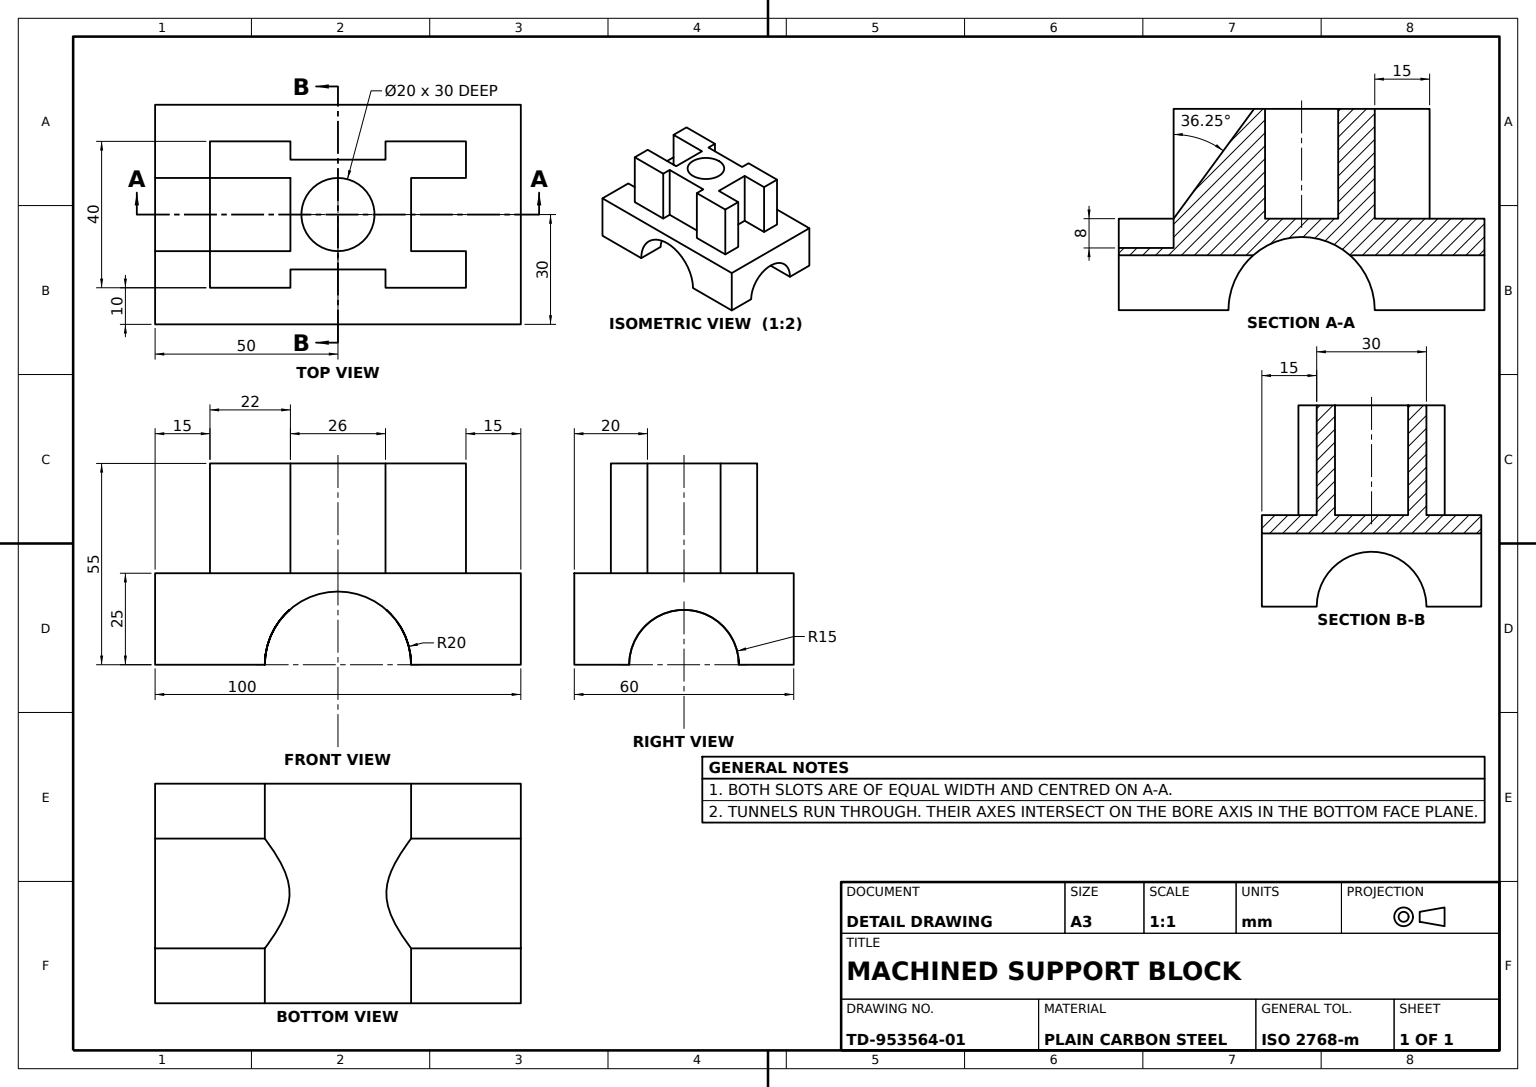
from build123d import *

# Parameters (mm, degrees)
SADDLE_BASE_BLOCK_DEPTH     = 30
THROUGH_HOLE_15_DEPTH       = 106.148704224
SLOT_CUT_DEPTH              = 15
CROSS_BOSS_PROFILE_SKETCH_R = 10
CROSS_BOSS_DEPTH            = 30
UPPER_PAD_SKETCH_W          = 20
UPPER_PAD_SKETCH_H          = 30
UPPER_PAD_DEPTH             = 15
NOTCH_CUT_DEPTH             = 30
NOTCH_FILL_BOSS_DEPTH       = 10


with BuildPart() as part:
    # Base Arch Profile Sketch → Saddle Base Block (new, symmetric)
    with BuildSketch(Plane.XY):
        with BuildLine():
            Line((20, -12.5), (50, -12.5))
            Line((50, -12.5), (50, 12.5))
            Line((50, 12.5), (-50, 12.5))
            Line((-50, 12.5), (-50, -12.5))
            Line((-50, -12.5), (-20, -12.5))
            ThreePointArc((-20, -12.5), (0, 7.5), (20, -12.5))
        make_face()
    extrude(amount=SADDLE_BASE_BLOCK_DEPTH, both=True)

    # Through Hole Sketch → Through Hole Ø15 (cut, through all)
    with BuildSketch(Plane.ZY.offset(50)):
        with BuildLine():
            Line((-15, -12.5), (15, -12.5))
            ThreePointArc((15, -12.5), (0, 2.5), (-15, -12.5))
        make_face()
    extrude(amount=-THROUGH_HOLE_15_DEPTH, mode=Mode.SUBTRACT)

    # Slot Profile Sketch → Slot Cut (cut)
    with BuildSketch(Plane.ZY.offset(50)):
        Polygon((0, 12.5), (10, 12.5), (10, 4.5), (-10, 4.5), (-10, 12.5), align=None)
    extrude(amount=-SLOT_CUT_DEPTH, mode=Mode.SUBTRACT)

    # Cross Boss Profile Sketch → Cross Boss (add)
    with BuildSketch(Plane(origin=(0, 12.5, 0), x_dir=(1, 0, 0), z_dir=(0, 1, 0))):
        Polygon((20, -10), (20, 10), (35, 10), (35, 20), (13, 20), (13, 15), (-13, 15), (-13, 20), (-35, 20), (-35, 10), (-20, 10), (-20, -10), (-35, -10), (-35, -20), (-13, -20), (-13, -15), (13, -15), (13, -20), (35, -20), (35, -10), align=None)
        with Locations(Location((0, 0, 0), (0, 0, 270))):
            Circle(CROSS_BOSS_PROFILE_SKETCH_R, mode=Mode.SUBTRACT)
    extrude(amount=CROSS_BOSS_DEPTH)

    # Upper Pad Sketch → Upper Pad (add)
    with BuildSketch(Plane.ZY.offset(20)):
        with Locations((0, 27.5)):
            Rectangle(UPPER_PAD_SKETCH_W, UPPER_PAD_SKETCH_H)
    extrude(amount=UPPER_PAD_DEPTH)

    # Notch Cut Sketch → Notch Cut (cut)
    with BuildSketch(Plane.XY.offset(20)):
        Polygon((-35, 12.5), (-13, 42.5), (-35, 42.5), align=None)
    extrude(amount=-NOTCH_CUT_DEPTH, mode=Mode.SUBTRACT)

    # Notch Fill Sketch → Notch Fill Boss (add)
    with BuildSketch(Plane.XY.offset(20)):
        Polygon((-35, 12.5), (-35, 42.5), (-13, 42.5), align=None)
    extrude(amount=-NOTCH_FILL_BOSS_DEPTH)


solid = part.part
